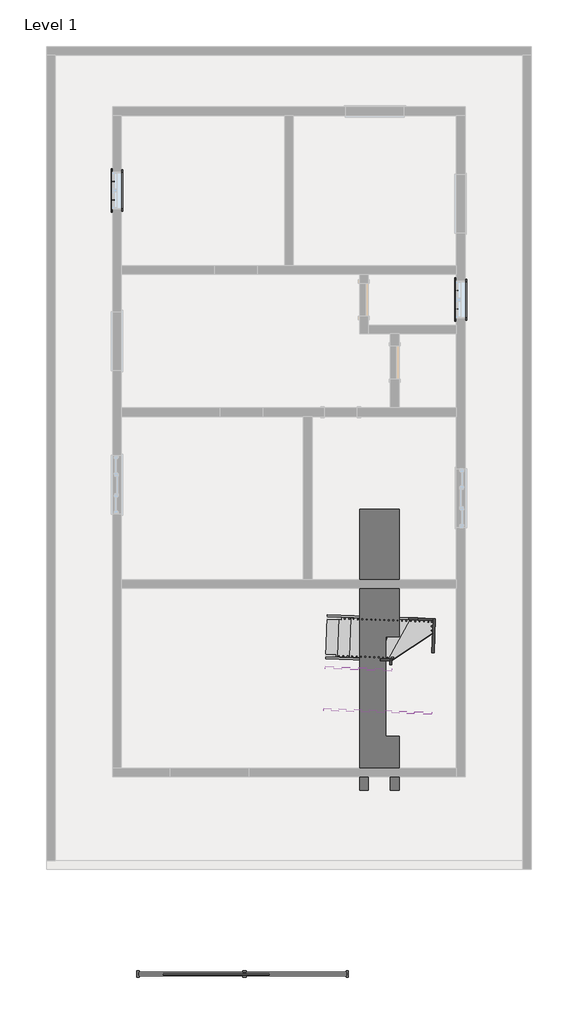
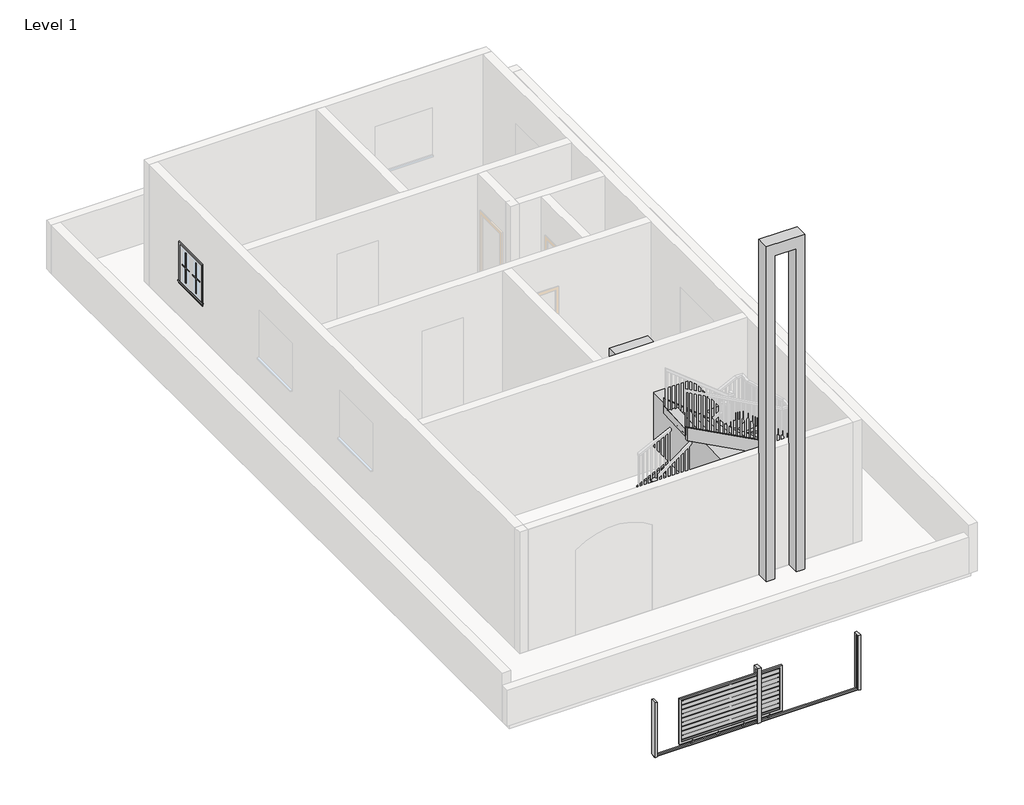
# One storey, part 4 of 4: 18 proxies, 16 members, 2 stair flights, 1 geographic element, 1 railing.
"""IFC4 building model written with IfcOpenShell, lengths in millimetres."""

from ifc_helpers import new_model, si_unit, frame, origin, place, context, project, spatial, polyline, outline, extrude, faceted_brep, transform, mapped, element, save
from components import generic_models_1_generic_models_1_9f30b8ca, generic_models_2_generic_models_2_975c2898, muntin_pattern_2x2_muntin_pattern_2x2_b3fe6957, muntin_pattern_2x2_muntin_pattern_2x2_3e0ecaf2, trim_window_exterior_flat_with_sill_41619996, trim_window_interior_flat_picture_frame_51c85655, sliding_gate_17236_sliding_gate_17236_fdb57db6, stair_flight_9054a24f

model = new_model("IFC4")

# Units and contexts
model_context = context("Model", 3, world=origin())
ifc_project = project(units=[si_unit("LENGTHUNIT", "METRE", prefix="MILLI")], contexts=[model_context])

# Site, building, storey
site = spatial("IfcSite", under=ifc_project)
building = spatial("IfcBuilding", under=site)
storey = spatial("IfcBuildingStorey", under=building, Name="Level 1", Elevation=0.0)

# Proxies
placement = place(None, origin())
generic_models_1_generic_models_1_shape = generic_models_1_generic_models_1_9f30b8ca(model_context)
element("IfcBuildingElementProxy", 1, Name="Generic Models 1 : Generic Models 1", ObjectType="Generic Models 1 : Generic Models 1", at=placement, inside=storey, context=model_context, shape_type="MappedRepresentation", body=[
    mapped(generic_models_1_generic_models_1_shape, transform((0.0, 0.0, 0.0), x_axis=(1.0, 0.0, 0.0), y_axis=(0.0, 1.0, 0.0), z_axis=(0.0, 0.0, 1.0))),
])
generic_models_2_generic_models_2_shape = generic_models_2_generic_models_2_975c2898(model_context)
element("IfcBuildingElementProxy", 2, Name="Generic Models 2 : Generic Models 2", ObjectType="Generic Models 2 : Generic Models 2", at=placement, inside=storey, context=model_context, shape_type="MappedRepresentation", body=[
    mapped(generic_models_2_generic_models_2_shape, transform((0.0, 0.0, 0.0), x_axis=(1.0, 0.0, 0.0), y_axis=(0.0, 1.0, 0.0), z_axis=(0.0, 0.0, 1.0))),
])
muntin_pattern_2x2_muntin_pattern_2x2_shape = muntin_pattern_2x2_muntin_pattern_2x2_b3fe6957(model_context)
element("IfcBuildingElementProxy", 3, Name="Muntin Pattern_2x2 : Muntin Pattern_2x2", ObjectType="Muntin Pattern_2x2 : Muntin Pattern_2x2", at=placement, inside=storey, context=model_context, shape_type="MappedRepresentation", body=[
    mapped(muntin_pattern_2x2_muntin_pattern_2x2_shape, transform((-14939.9876504, 9248.016357, 984.25), x_axis=(0.0, 1.0, 0.0), y_axis=(-1.0, 0.0, 0.0), z_axis=(0.0, 0.0, 1.0))),
])
element("IfcBuildingElementProxy", 4, Name="Muntin Pattern_2x2 : Muntin Pattern_2x2", ObjectType="Muntin Pattern_2x2 : Muntin Pattern_2x2", at=placement, inside=storey, context=model_context, shape_type="MappedRepresentation", body=[
    mapped(muntin_pattern_2x2_muntin_pattern_2x2_shape, transform((-7015.1876504, 6733.416357, 984.25), x_axis=(0.0, 1.0, 0.0), y_axis=(-1.0, 0.0, 0.0), z_axis=(0.0, 0.0, 1.0))),
])
element("IfcBuildingElementProxy", 5, Name="Muntin Pattern_2x2 : Muntin Pattern_2x2", ObjectType="Muntin Pattern_2x2 : Muntin Pattern_2x2", at=placement, inside=storey, context=model_context, shape_type="MappedRepresentation", body=[
    mapped(muntin_pattern_2x2_muntin_pattern_2x2_shape, transform((-14939.9876504, 9248.016357, 984.25), x_axis=(0.0, 1.0, 0.0), y_axis=(-1.0, 0.0, 0.0), z_axis=(0.0, 0.0, 1.0))),
])
element("IfcBuildingElementProxy", 6, Name="Muntin Pattern_2x2 : Muntin Pattern_2x2", ObjectType="Muntin Pattern_2x2 : Muntin Pattern_2x2", at=placement, inside=storey, context=model_context, shape_type="MappedRepresentation", body=[
    mapped(muntin_pattern_2x2_muntin_pattern_2x2_shape, transform((-7015.1876504, 6733.416357, 984.25), x_axis=(0.0, 1.0, 0.0), y_axis=(-1.0, 0.0, 0.0), z_axis=(0.0, 0.0, 1.0))),
])
muntin_pattern_2x2_muntin_pattern_2x2_2_shape = muntin_pattern_2x2_muntin_pattern_2x2_3e0ecaf2(model_context)
element("IfcBuildingElementProxy", 7, Name="Muntin Pattern_2x2 : Muntin Pattern_2x2", ObjectType="Muntin Pattern_2x2 : Muntin Pattern_2x2", at=placement, inside=storey, context=model_context, shape_type="MappedRepresentation", body=[
    mapped(muntin_pattern_2x2_muntin_pattern_2x2_2_shape, transform((-14939.9876504, 9676.641357, 984.25), x_axis=(0.0, -1.0, 0.0), y_axis=(1.0, 0.0, 0.0), z_axis=(0.0, 0.0, 1.0))),
])
element("IfcBuildingElementProxy", 8, Name="Muntin Pattern_2x2 : Muntin Pattern_2x2", ObjectType="Muntin Pattern_2x2 : Muntin Pattern_2x2", at=placement, inside=storey, context=model_context, shape_type="MappedRepresentation", body=[
    mapped(muntin_pattern_2x2_muntin_pattern_2x2_2_shape, transform((-7015.1876504, 7162.041357, 984.25), x_axis=(0.0, -1.0, 0.0), y_axis=(1.0, 0.0, 0.0), z_axis=(0.0, 0.0, 1.0))),
])
element("IfcBuildingElementProxy", 9, Name="Muntin Pattern_2x2 : Muntin Pattern_2x2", ObjectType="Muntin Pattern_2x2 : Muntin Pattern_2x2", at=placement, inside=storey, context=model_context, shape_type="MappedRepresentation", body=[
    mapped(muntin_pattern_2x2_muntin_pattern_2x2_2_shape, transform((-14939.9876504, 9676.641357, 984.25), x_axis=(0.0, -1.0, 0.0), y_axis=(1.0, 0.0, 0.0), z_axis=(0.0, 0.0, 1.0))),
])
element("IfcBuildingElementProxy", 10, Name="Muntin Pattern_2x2 : Muntin Pattern_2x2", ObjectType="Muntin Pattern_2x2 : Muntin Pattern_2x2", at=placement, inside=storey, context=model_context, shape_type="MappedRepresentation", body=[
    mapped(muntin_pattern_2x2_muntin_pattern_2x2_2_shape, transform((-7015.1876504, 7162.041357, 984.25), x_axis=(0.0, -1.0, 0.0), y_axis=(1.0, 0.0, 0.0), z_axis=(0.0, 0.0, 1.0))),
])
trim_window_exterior_flat_with_sill_shape = trim_window_exterior_flat_with_sill_41619996(model_context)
element("IfcBuildingElementProxy", 11, Name="Trim-Window-Exterior-Flat : with Sill", ObjectType="Trim-Window-Exterior-Flat : with Sill", at=placement, inside=storey, context=model_context, shape_type="MappedRepresentation", body=[
    mapped(trim_window_exterior_flat_with_sill_shape, transform((-14949.5126504, 9462.328857, 1828.8), x_axis=(0.0, -1.0, 0.0), y_axis=(0.0, 0.0, 1.0), z_axis=(-1.0, 0.0, 0.0))),
])
element("IfcBuildingElementProxy", 12, Name="Trim-Window-Exterior-Flat : with Sill", ObjectType="Trim-Window-Exterior-Flat : with Sill", at=placement, inside=storey, context=model_context, shape_type="MappedRepresentation", body=[
    mapped(trim_window_exterior_flat_with_sill_shape, transform((-7024.7126504, 6947.728857, 1828.8), x_axis=(0.0, -1.0, 0.0), y_axis=(0.0, 0.0, 1.0), z_axis=(-1.0, 0.0, 0.0))),
])
element("IfcBuildingElementProxy", 13, Name="Trim-Window-Exterior-Flat : with Sill", ObjectType="Trim-Window-Exterior-Flat : with Sill", at=placement, inside=storey, context=model_context, shape_type="MappedRepresentation", body=[
    mapped(trim_window_exterior_flat_with_sill_shape, transform((-14949.5126504, 9462.328857, 1828.8), x_axis=(0.0, -1.0, 0.0), y_axis=(0.0, 0.0, 1.0), z_axis=(-1.0, 0.0, 0.0))),
])
element("IfcBuildingElementProxy", 14, Name="Trim-Window-Exterior-Flat : with Sill", ObjectType="Trim-Window-Exterior-Flat : with Sill", at=placement, inside=storey, context=model_context, shape_type="MappedRepresentation", body=[
    mapped(trim_window_exterior_flat_with_sill_shape, transform((-7024.7126504, 6947.728857, 1828.8), x_axis=(0.0, -1.0, 0.0), y_axis=(0.0, 0.0, 1.0), z_axis=(-1.0, 0.0, 0.0))),
])
trim_window_interior_flat_picture_frame_shape = trim_window_interior_flat_picture_frame_51c85655(model_context)
element("IfcBuildingElementProxy", 15, Name="Trim-Window-Interior-Flat : Picture Frame", ObjectType="Trim-Window-Interior-Flat : Picture Frame", at=placement, inside=storey, context=model_context, shape_type="MappedRepresentation", body=[
    mapped(trim_window_interior_flat_picture_frame_shape, transform((-14746.3126504, 9462.328857, 1828.8), x_axis=(0.0, 1.0, 0.0), y_axis=(0.0, 0.0, 1.0), z_axis=(1.0, 0.0, 0.0))),
])
element("IfcBuildingElementProxy", 16, Name="Trim-Window-Interior-Flat : Picture Frame", ObjectType="Trim-Window-Interior-Flat : Picture Frame", at=placement, inside=storey, context=model_context, shape_type="MappedRepresentation", body=[
    mapped(trim_window_interior_flat_picture_frame_shape, transform((-6821.5126504, 6947.728857, 1828.8), x_axis=(0.0, 1.0, 0.0), y_axis=(0.0, 0.0, 1.0), z_axis=(1.0, 0.0, 0.0))),
])
element("IfcBuildingElementProxy", 17, Name="Trim-Window-Interior-Flat : Picture Frame", ObjectType="Trim-Window-Interior-Flat : Picture Frame", at=placement, inside=storey, context=model_context, shape_type="MappedRepresentation", body=[
    mapped(trim_window_interior_flat_picture_frame_shape, transform((-14746.3126504, 9462.328857, 1828.8), x_axis=(0.0, 1.0, 0.0), y_axis=(0.0, 0.0, 1.0), z_axis=(1.0, 0.0, 0.0))),
])
element("IfcBuildingElementProxy", 18, Name="Trim-Window-Interior-Flat : Picture Frame", ObjectType="Trim-Window-Interior-Flat : Picture Frame", at=placement, inside=storey, context=model_context, shape_type="MappedRepresentation", body=[
    mapped(trim_window_interior_flat_picture_frame_shape, transform((-6821.5126504, 6947.728857, 1828.8), x_axis=(0.0, 1.0, 0.0), y_axis=(0.0, 0.0, 1.0), z_axis=(1.0, 0.0, 0.0))),
])

# Geographic element
sliding_gate_17236_sliding_gate_17236_shape = sliding_gate_17236_sliding_gate_17236_fdb57db6(model_context)
element("IfcGeographicElement", 19, ObjectType="Sliding_Gate_17236 : Sliding_Gate_17236", at=placement, inside=storey, context=model_context, shape_type="MappedRepresentation", body=[
    mapped(sliding_gate_17236_sliding_gate_17236_shape, transform((-14390.7126504, -8673.271143, 0.0), x_axis=(1.0, 0.0, 0.0), y_axis=(0.0, 1.0, 0.0), z_axis=(0.0, 0.0, 1.0))),
])

# Members
element("IfcMember", 20, ObjectType="Stringer - 2\" Width", at=placement, inside=storey, context=model_context, shape_type="SweptSolid", body=[
    extrude(outline(polyline([(157.0794453, -304.8), (51.8818925, -100.6726296), (247.2290139, 0.0), (2348.3102094, 0.0), (2505.3896547, -304.8), (157.0794453, -304.8)])), frame((-10006.394185, -363.3128759, -113.2550622), z_axis=(0.03595828761805287, 0.9993532916599501, 0.0), x_axis=(0.8883269481492083, -0.03196338688929392, 0.45809777896261317)), (0.0, 0.0, 1.0), 50.8),
])
element("IfcMember", 21, ObjectType="Stringer - 2\" Width", at=placement, inside=storey, context=model_context, shape_type="SweptSolid", body=[
    extrude(outline(polyline([(-7920.3269434, -438.3728236), (-7918.5002624, -387.6056764), (-7564.0151591, -400.3606025), (-7565.8418401, -451.1277497), (-7920.3269434, -438.3728236)])), frame((0.0, 0.0, 962.500629), z_axis=(0.0, 0.0, 1.0), x_axis=(1.0, 0.0, 0.0)), (0.0, 0.0, 1.0), 342.8950162),
])
element("IfcMember", 22, ObjectType="Stringer - 2\" Width", at=placement, inside=storey, context=model_context, shape_type="SweptSolid", body=[
    extrude(outline(polyline([(-141.4966894, -274.7041443), (-53.351137, 0.0), (2175.2349578, 0.0), (2210.4467651, -11.2985708), (2109.3071449, -326.4985112), (19.9195916, -326.4985112), (-141.4966894, -274.7041443)])), frame((-7515.0746928, -452.9544307, 1305.3956453), z_axis=(-0.9993532916599502, 0.035958287618053086, 0.0), x_axis=(-0.034238839346999, -0.9515663584286188, 0.30553095978487654)), (0.0, 0.0, 1.0), 50.8),
])
element("IfcMember", 23, ObjectType="Stringer - 2\" Width", at=placement, inside=storey, context=model_context, shape_type="SweptSolid", body=[
    extrude(outline(polyline([(-7590.8819548, -2559.7910402), (-7592.7086358, -2610.5581874), (-7997.9608864, -2595.9765803), (-7996.1342054, -2545.2094331), (-7590.8819548, -2559.7910402)])), frame((0.0, 0.0, 1649.8904473), z_axis=(0.0, 0.0, 1.0), x_axis=(1.0, 0.0, 0.0)), (0.0, 0.0, 1.0), 320.1068224),
])
element("IfcMember", 24, ObjectType="Stringer - 2\" Width", at=placement, inside=storey, context=model_context, shape_type="SweptSolid", body=[
    extrude(outline(polyline([(-146.6402244, -284.5435333), (0.0, 0.0), (2348.3102094, 0.0), (2201.669985, -284.5435333), (-146.6402244, -284.5435333)])), frame((-7997.9608864, -2595.9765803, 1969.9972697), z_axis=(0.03595828761805282, 0.9993532916599503, 0.0), x_axis=(-0.8883269481492089, 0.031963386889293885, 0.45809777896261206)), (0.0, 0.0, 1.0), 50.8),
])
element("IfcMember", 25, ObjectType="Stringer - 2\" Width", at=placement, inside=storey, context=model_context, shape_type="SweptSolid", body=[
    extrude(outline(polyline([(248.5240347, -304.8), (137.1927864, -168.2588219), (343.5522597, 0.0), (1905.6564494, 0.0), (2154.1804842, -304.8), (248.5240347, -304.8)])), frame((-10041.1011242, -1327.888673, -217.1011096), z_axis=(0.03595828761805293, 0.9993532916599501, 0.0), x_axis=(0.7745239433168307, -0.02786857756239004, 0.6319303787709498)), (0.0, 0.0, 1.0), 50.8),
])
element("IfcMember", 26, ObjectType="Stringer - 2\" Width", at=placement, inside=storey, context=model_context, shape_type="SweptSolid", body=[
    extrude(outline(polyline([(-470.0446027, -275.2513009), (0.0, 0.0), (408.9230004, 1e-07), (420.0212921, -18.9524702), (-68.1184117, -304.7999999), (-452.7413132, -304.8), (-470.0446027, -275.2513009)])), frame((-8512.5307482, -1332.0561414, 1573.2682978), z_axis=(-0.9993532916599503, 0.03595828761805069, 0.0), x_axis=(-0.01817045481332337, -0.5049935642524205, 0.8629318250218342)), (0.0, 0.0, 1.0), 50.8),
])
element("IfcMember", 27, ObjectType="Stringer - 2\" Width", at=placement, inside=storey, context=model_context, shape_type="SweptSolid", body=[
    extrude(outline(polyline([(-248.5240348, -304.8), (0.0, 0.0), (1971.2027087, 0.0), (1722.6786739, -304.8), (-248.5240348, -304.8)])), frame((-8522.5774937, -1611.2754511, 1926.1409689), z_axis=(0.0359582876180528, 0.9993532916599502, 0.0), x_axis=(-0.7745239433168302, 0.027868577562389925, 0.6319303787709503)), (0.0, 0.0, 1.0), 50.8),
])
element("IfcMember", 28, ObjectType="Stringer - 2\" Width", at=placement, inside=storey, context=model_context, shape_type="SweptSolid", body=[
    extrude(outline(polyline([(157.0794453, -304.8), (51.8818925, -100.6726296), (247.2290139, 0.0), (2348.3102094, 0.0), (2505.3896547, -304.8), (157.0794453, -304.8)])), frame((-10006.394185, -363.3128759, -113.2550622), z_axis=(0.03595828761805287, 0.9993532916599501, 0.0), x_axis=(0.8883269481492083, -0.03196338688929392, 0.45809777896261317)), (0.0, 0.0, 1.0), 50.8),
])
element("IfcMember", 29, ObjectType="Stringer - 2\" Width", at=placement, inside=storey, context=model_context, shape_type="SweptSolid", body=[
    extrude(outline(polyline([(-7920.3269434, -438.3728236), (-7918.5002624, -387.6056764), (-7564.0151591, -400.3606025), (-7565.8418401, -451.1277497), (-7920.3269434, -438.3728236)])), frame((0.0, 0.0, 962.500629), z_axis=(0.0, 0.0, 1.0), x_axis=(1.0, 0.0, 0.0)), (0.0, 0.0, 1.0), 342.8950162),
])
element("IfcMember", 30, ObjectType="Stringer - 2\" Width", at=placement, inside=storey, context=model_context, shape_type="SweptSolid", body=[
    extrude(outline(polyline([(-141.4966894, -274.7041443), (-53.351137, 0.0), (2175.2349578, 0.0), (2210.4467651, -11.2985708), (2109.3071449, -326.4985112), (19.9195916, -326.4985112), (-141.4966894, -274.7041443)])), frame((-7515.0746928, -452.9544307, 1305.3956453), z_axis=(-0.9993532916599502, 0.035958287618053086, 0.0), x_axis=(-0.034238839346999, -0.9515663584286188, 0.30553095978487654)), (0.0, 0.0, 1.0), 50.8),
])
element("IfcMember", 31, ObjectType="Stringer - 2\" Width", at=placement, inside=storey, context=model_context, shape_type="SweptSolid", body=[
    extrude(outline(polyline([(-7590.8819548, -2559.7910402), (-7592.7086358, -2610.5581874), (-7997.9608864, -2595.9765803), (-7996.1342054, -2545.2094331), (-7590.8819548, -2559.7910402)])), frame((0.0, 0.0, 1649.8904473), z_axis=(0.0, 0.0, 1.0), x_axis=(1.0, 0.0, 0.0)), (0.0, 0.0, 1.0), 320.1068224),
])
element("IfcMember", 32, ObjectType="Stringer - 2\" Width", at=placement, inside=storey, context=model_context, shape_type="SweptSolid", body=[
    extrude(outline(polyline([(-146.6402244, -284.5435333), (0.0, 0.0), (2348.3102094, 0.0), (2201.669985, -284.5435333), (-146.6402244, -284.5435333)])), frame((-7997.9608864, -2595.9765803, 1969.9972697), z_axis=(0.03595828761805282, 0.9993532916599503, 0.0), x_axis=(-0.8883269481492089, 0.031963386889293885, 0.45809777896261206)), (0.0, 0.0, 1.0), 50.8),
])
element("IfcMember", 33, ObjectType="Stringer - 2\" Width", at=placement, inside=storey, context=model_context, shape_type="SweptSolid", body=[
    extrude(outline(polyline([(248.5240347, -304.8), (137.1927864, -168.2588219), (343.5522597, 0.0), (1905.6564494, 0.0), (2154.1804842, -304.8), (248.5240347, -304.8)])), frame((-10041.1011242, -1327.888673, -217.1011096), z_axis=(0.03595828761805293, 0.9993532916599501, 0.0), x_axis=(0.7745239433168307, -0.02786857756239004, 0.6319303787709498)), (0.0, 0.0, 1.0), 50.8),
])
element("IfcMember", 34, ObjectType="Stringer - 2\" Width", at=placement, inside=storey, context=model_context, shape_type="SweptSolid", body=[
    extrude(outline(polyline([(-470.0446027, -275.2513009), (0.0, 0.0), (408.9230004, 1e-07), (420.0212921, -18.9524702), (-68.1184117, -304.7999999), (-452.7413132, -304.8), (-470.0446027, -275.2513009)])), frame((-8512.5307482, -1332.0561414, 1573.2682978), z_axis=(-0.9993532916599503, 0.03595828761805069, 0.0), x_axis=(-0.01817045481332337, -0.5049935642524205, 0.8629318250218342)), (0.0, 0.0, 1.0), 50.8),
])
element("IfcMember", 35, ObjectType="Stringer - 2\" Width", at=placement, inside=storey, context=model_context, shape_type="SweptSolid", body=[
    extrude(outline(polyline([(-248.5240348, -304.8), (0.0, 0.0), (1971.2027087, 0.0), (1722.6786739, -304.8), (-248.5240348, -304.8)])), frame((-8522.5774937, -1611.2754511, 1926.1409689), z_axis=(0.0359582876180528, 0.9993532916599502, 0.0), x_axis=(-0.7745239433168302, 0.027868577562389925, 0.6319303787709503)), (0.0, 0.0, 1.0), 50.8),
])

# Railing
element("IfcRailing", 36, ObjectType="Handrail - Rectangular", at=placement, inside=storey, context=model_context, shape_type="SolidModel", body=[
    faceted_brep([(-10006.394185, -363.3128759, 1083.7333333), (-10006.394185, -363.3128759, 1026.2742652), (-10008.220866, -414.0800231, 1026.2742652), (-10008.220866, -414.0800231, 1083.7333333), (-7750.1292126, -444.496803, 2277.0239201), (-7737.5382959, -444.9498438, 2226.2239201), (-7739.364977, -495.716991, 2226.2239201), (-7751.9558936, -495.2639503, 2277.0239201), (-7565.8418401, -451.1277497, 2277.0239201), (-7565.8418401, -451.1277497, 2226.2239201), (-7618.4356683, -500.0682159, 2226.2239201), (-7618.4356683, -500.0682159, 2277.0239201), (-7576.1730834, -738.2538248, 2277.0239201), (-7576.4589725, -746.1992592, 2226.2239201), (-7627.2261197, -744.3725782, 2226.2239201), (-7626.9402306, -736.4271438, 2277.0239201), (-7631.3178587, -2270.838284, 2769.1094132), (-7631.6037478, -2278.7837184, 2718.3094132), (-7682.370895, -2276.9570374, 2718.3094132), (-7682.0850059, -2269.011603, 2769.1094132), (-7641.649102, -2557.9643591, 2769.1094132), (-7641.649102, -2557.9643591, 2718.3094132), (-7690.5895682, -2505.3705309, 2718.3094132), (-7690.5895682, -2505.3705309, 2769.1094132), (-7825.9364745, -2551.3334125, 2769.1094132), (-7838.5273911, -2550.8803717, 2718.3094132), (-7836.7007101, -2500.1132245, 2718.3094132), (-7824.1097935, -2500.5662653, 2769.1094132), (-10082.2014469, -2470.1494854, 3962.4), (-10080.3747659, -2419.3823382, 3962.4), (-10080.3747659, -2419.3823382, 3904.9409318), (-10082.2014469, -2470.1494854, 3904.9409318)], [[[0, 1, 2, 3]], [[1, 0, 4, 5]], [[2, 1, 5, 6]], [[3, 2, 6, 7]], [[0, 3, 7, 4]], [[5, 4, 8, 9]], [[6, 5, 9, 10]], [[7, 6, 10, 11]], [[4, 7, 11, 8]], [[9, 8, 12, 13]], [[10, 9, 13, 14]], [[11, 10, 14, 15]], [[8, 11, 15, 12]], [[13, 12, 16, 17]], [[14, 13, 17, 18]], [[15, 14, 18, 19]], [[12, 15, 19, 16]], [[17, 16, 20, 21]], [[18, 17, 21, 22]], [[19, 18, 22, 23]], [[16, 19, 23, 20]], [[21, 20, 24, 25]], [[22, 21, 25, 26]], [[23, 22, 26, 27]], [[20, 23, 27, 24]], [[28, 29, 30, 31]], [[25, 24, 28, 31]], [[26, 25, 31, 30]], [[27, 26, 30, 29]], [[24, 27, 29, 28]]]),
    extrude(outline(polyline([(223.5656878, 19.05), (1212.6274313, 19.05), (1212.6274313, 0.0), (233.6343122, 0.0), (223.5656878, 19.05)])), frame((-9992.2317697, -2457.5014613, 4091.294098), z_axis=(0.035958287618052934, 0.9993532916599503, 0.0), x_axis=(0.0, 0.0, -1.0)), (0.0, 0.0, 1.0), 19.05),
    extrude(outline(polyline([(223.5656878, 19.05), (1158.9281011, 19.05), (1158.9281011, 0.0), (233.6343122, 0.0), (223.5656878, 19.05)])), frame((-9890.6974752, -2461.1548233, 4037.5947678), z_axis=(0.035958287618052934, 0.9993532916599503, 0.0), x_axis=(0.0, 0.0, -1.0)), (0.0, 0.0, 1.0), 19.05),
    extrude(outline(polyline([(223.5656878, 19.05), (1274.5621043, 19.05), (1274.5621043, 0.0), (233.6343122, 0.0), (223.5656878, 19.05)])), frame((-9789.1631808, -2464.8081854, 3983.8954376), z_axis=(0.035958287618052934, 0.9993532916599503, 0.0), x_axis=(0.0, 0.0, -1.0)), (0.0, 0.0, 1.0), 19.05),
    extrude(outline(polyline([(223.5656878, 19.05), (1220.8627741, 19.05), (1220.8627741, 0.0), (233.6343122, 0.0), (223.5656878, 19.05)])), frame((-9687.6288864, -2468.4615474, 3930.1961074), z_axis=(0.035958287618052934, 0.9993532916599503, 0.0), x_axis=(0.0, 0.0, -1.0)), (0.0, 0.0, 1.0), 19.05),
    extrude(outline(polyline([(223.5656878, 19.05), (1167.1634439, 19.05), (1167.1634439, 0.0), (233.6343122, 0.0), (223.5656878, 19.05)])), frame((-9586.0945919, -2472.1149094, 3876.4967772), z_axis=(0.035958287618052934, 0.9993532916599503, 0.0), x_axis=(0.0, 0.0, -1.0)), (0.0, 0.0, 1.0), 19.05),
    extrude(outline(polyline([(223.5656878, 19.05), (1282.797447, 19.05), (1282.797447, 0.0), (233.6343122, 0.0), (223.5656878, 19.05)])), frame((-9484.5602975, -2475.7682714, 3822.797447), z_axis=(0.035958287618052934, 0.9993532916599503, 0.0), x_axis=(0.0, 0.0, -1.0)), (0.0, 0.0, 1.0), 19.05),
    extrude(outline(polyline([(223.5656878, 19.05), (1229.0981168, 19.05), (1229.0981168, 0.0), (233.6343122, 0.0), (223.5656878, 19.05)])), frame((-9383.0260031, -2479.4216334, 3769.0981168), z_axis=(0.035958287618052934, 0.9993532916599503, 0.0), x_axis=(0.0, 0.0, -1.0)), (0.0, 0.0, 1.0), 19.05),
    extrude(outline(polyline([(223.5656878, 19.05), (1175.3987866, 19.05), (1175.3987866, 0.0), (233.6343122, 0.0), (223.5656878, 19.05)])), frame((-9281.4917086, -2483.0749955, 3715.3987866), z_axis=(0.035958287618052934, 0.9993532916599503, 0.0), x_axis=(0.0, 0.0, -1.0)), (0.0, 0.0, 1.0), 19.05),
    extrude(outline(polyline([(223.5656878, 19.05), (1291.0327897, 19.05), (1291.0327897, 0.0), (233.6343122, 0.0), (223.5656878, 19.05)])), frame((-9179.9574142, -2486.7283575, 3661.6994564), z_axis=(0.035958287618052934, 0.9993532916599503, 0.0), x_axis=(0.0, 0.0, -1.0)), (0.0, 0.0, 1.0), 19.05),
    extrude(outline(polyline([(223.5656878, 19.05), (1237.3334595, 19.05), (1237.3334595, 0.0), (233.6343122, 0.0), (223.5656878, 19.05)])), frame((-9078.4231198, -2490.3817195, 3608.0001262), z_axis=(0.035958287618052934, 0.9993532916599503, 0.0), x_axis=(0.0, 0.0, -1.0)), (0.0, 0.0, 1.0), 19.05),
    extrude(outline(polyline([(223.5656878, 19.05), (1183.6341293, 19.05), (1183.6341293, 0.0), (233.6343122, 0.0), (223.5656878, 19.05)])), frame((-8976.8888253, -2494.0350815, 3554.300796), z_axis=(0.035958287618052934, 0.9993532916599503, 0.0), x_axis=(0.0, 0.0, -1.0)), (0.0, 0.0, 1.0), 19.05),
    extrude(outline(polyline([(223.5656878, 19.05), (1299.2681325, 19.05), (1299.2681325, 0.0), (233.6343122, 0.0), (223.5656878, 19.05)])), frame((-8875.3545309, -2497.6884436, 3500.6014658), z_axis=(0.035958287618052934, 0.9993532916599503, 0.0), x_axis=(0.0, 0.0, -1.0)), (0.0, 0.0, 1.0), 19.05),
    extrude(outline(polyline([(223.5656878, 19.05), (1245.5688023, 19.05), (1245.5688023, 0.0), (233.6343122, 0.0), (223.5656878, 19.05)])), frame((-8773.8202365, -2501.3418056, 3446.9021356), z_axis=(0.035958287618052934, 0.9993532916599503, 0.0), x_axis=(0.0, 0.0, -1.0)), (0.0, 0.0, 1.0), 19.05),
    extrude(outline(polyline([(223.5656878, 19.05), (1191.8694721, 19.05), (1191.8694721, 0.0), (233.6343122, 0.0), (223.5656878, 19.05)])), frame((-8672.285942, -2504.9951676, 3393.2028054), z_axis=(0.035958287618052934, 0.9993532916599503, 0.0), x_axis=(0.0, 0.0, -1.0)), (0.0, 0.0, 1.0), 19.05),
    extrude(outline(polyline([(223.5656878, 19.05), (1138.1701419, 19.05), (1138.1701419, 0.0), (233.6343122, 0.0), (223.5656878, 19.05)])), frame((-8570.7516476, -2508.6485296, 3339.5034752), z_axis=(0.035958287618052934, 0.9993532916599503, 0.0), x_axis=(0.0, 0.0, -1.0)), (0.0, 0.0, 1.0), 19.05),
    extrude(outline(polyline([(223.5656878, 19.05), (1253.804145, 19.05), (1253.804145, 0.0), (233.6343122, 0.0), (223.5656878, 19.05)])), frame((-8469.2173532, -2512.3018916, 3285.804145), z_axis=(0.035958287618052934, 0.9993532916599503, 0.0), x_axis=(0.0, 0.0, -1.0)), (0.0, 0.0, 1.0), 19.05),
    extrude(outline(polyline([(223.5656878, 19.05), (1200.1048148, 19.05), (1200.1048148, 0.0), (233.6343122, 0.0), (223.5656878, 19.05)])), frame((-8367.6830587, -2515.9552537, 3232.1048148), z_axis=(0.035958287618052934, 0.9993532916599503, 0.0), x_axis=(0.0, 0.0, -1.0)), (0.0, 0.0, 1.0), 19.05),
    extrude(outline(polyline([(223.5656878, 19.05), (1146.4054846, 19.05), (1146.4054846, 0.0), (233.6343122, 0.0), (223.5656878, 19.05)])), frame((-8266.1487643, -2519.6086157, 3178.4054846), z_axis=(0.035958287618052934, 0.9993532916599503, 0.0), x_axis=(0.0, 0.0, -1.0)), (0.0, 0.0, 1.0), 19.05),
    extrude(outline(polyline([(223.5656878, 19.05), (1092.7061544, 19.05), (1092.7061544, 0.0), (233.6343122, 0.0), (223.5656878, 19.05)])), frame((-8164.6144699, -2523.2619777, 3124.7061544), z_axis=(0.035958287618052934, 0.9993532916599503, 0.0), x_axis=(0.0, 0.0, -1.0)), (0.0, 0.0, 1.0), 19.05),
    extrude(outline(polyline([(223.5656878, 19.05), (1208.3401575, 19.05), (1208.3401575, 0.0), (233.6343122, 0.0), (223.5656878, 19.05)])), frame((-8063.0801754, -2526.9153397, 3071.0068242), z_axis=(0.035958287618052934, 0.9993532916599503, 0.0), x_axis=(0.0, 0.0, -1.0)), (0.0, 0.0, 1.0), 19.05),
    extrude(outline(polyline([(223.5656878, 19.05), (1154.6408273, 19.05), (1154.6408273, 0.0), (233.6343122, 0.0), (223.5656878, 19.05)])), frame((-7961.545881, -2530.5687018, 3017.307494), z_axis=(0.035958287618052934, 0.9993532916599503, 0.0), x_axis=(0.0, 0.0, -1.0)), (0.0, 0.0, 1.0), 19.05),
    extrude(outline(polyline([(223.5656878, 19.05), (1100.9414971, 19.05), (1100.9414971, 0.0), (233.6343122, 0.0), (223.5656878, 19.05)])), frame((-7860.0115866, -2534.2220638, 2963.6081638), z_axis=(0.035958287618052934, 0.9993532916599503, 0.0), x_axis=(0.0, 0.0, -1.0)), (0.0, 0.0, 1.0), 19.05),
    extrude(outline(polyline([(-7758.4772921, -2537.8754258), (-7777.5149723, -2537.1904204), (-7776.829967, -2518.1527402), (-7757.7922868, -2518.8377456), (-7758.4772921, -2537.8754258)])), frame((0.0, 0.0, 1862.6666667), z_axis=(0.0, 0.0, 1.0), x_axis=(1.0, 0.0, 0.0)), (0.0, 0.0, 1.0), 855.6427466),
    extrude(outline(polyline([(-7655.3446518, -2497.107534), (-7656.0296572, -2516.1452142), (-7675.0673374, -2515.4602088), (-7674.382332, -2496.4225286), (-7655.3446518, -2497.107534)])), frame((0.0, 0.0, 1862.6666667), z_axis=(0.0, 0.0, 1.0), x_axis=(1.0, 0.0, 0.0)), (0.0, 0.0, 1.0), 855.6427466),
    extrude(outline(polyline([(-7651.6912898, -2395.5732396), (-7652.3762952, -2414.6109198), (-7671.4139754, -2413.9259144), (-7670.72897, -2394.8882342), (-7651.6912898, -2395.5732396)])), frame((0.0, 0.0, 1862.6666667), z_axis=(0.0, 0.0, 1.0), x_axis=(1.0, 0.0, 0.0)), (0.0, 0.0, 1.0), 855.6427466),
    extrude(outline(polyline([(-7648.0379278, -2294.0389451), (-7648.7229332, -2313.0766254), (-7667.7606134, -2312.39162), (-7667.075608, -2293.3539398), (-7648.0379278, -2294.0389451)])), frame((0.0, 0.0, 1862.6666667), z_axis=(0.0, 0.0, 1.0), x_axis=(1.0, 0.0, 0.0)), (0.0, 0.0, 1.0), 855.6427466),
    extrude(outline(polyline([(225.5436705, 19.05), (1229.1130279, 19.05), (1229.1130279, 0.0), (231.6563296, 0.0), (225.5436705, 19.05)])), frame((-7644.3845658, -2192.5046507, 2922.4463612), z_axis=(-0.9993532916599501, 0.03595828761805307, 0.0), x_axis=(0.0, 0.0, -1.0)), (0.0, 0.0, 1.0), 19.05),
    extrude(outline(polyline([(225.5436704, 19.05), (1196.5121796, 19.05), (1196.5121796, 0.0), (231.6563295, 0.0), (225.5436704, 19.05)])), frame((-7640.7312037, -2090.9703563, 2889.8455129), z_axis=(-0.9993532916599501, 0.03595828761805307, 0.0), x_axis=(0.0, 0.0, -1.0)), (0.0, 0.0, 1.0), 19.05),
    extrude(outline(polyline([(225.5436705, 19.0500001), (1163.9113314, 19.0500001), (1163.9113314, 0.0), (231.6563295, 0.0), (225.5436705, 19.0500001)])), frame((-7637.0778417, -1989.4360618, 2857.2446647), z_axis=(-0.9993532916599501, 0.03595828761805307, 0.0), x_axis=(0.0, 0.0, -1.0)), (0.0, 0.0, 1.0), 19.05),
    extrude(outline(polyline([(225.5436705, 19.05), (1131.3104832, 19.05), (1131.3104832, 0.0), (231.6563295, 0.0), (225.5436705, 19.05)])), frame((-7633.4244797, -1887.9017674, 2824.6438165), z_axis=(-0.9993532916599501, 0.03595828761805307, 0.0), x_axis=(0.0, 0.0, -1.0)), (0.0, 0.0, 1.0), 19.05),
    extrude(outline(polyline([(225.5436705, 19.05), (1098.709635, 19.05), (1098.709635, 0.0), (231.6563296, 0.0), (225.5436705, 19.05)])), frame((-7629.7711177, -1786.367473, 2792.0429683), z_axis=(-0.9993532916599501, 0.03595828761805307, 0.0), x_axis=(0.0, 0.0, -1.0)), (0.0, 0.0, 1.0), 19.05),
    extrude(outline(polyline([(225.5436705, 19.0500001), (1235.44212, 19.0500001), (1235.44212, 0.0), (231.6563295, 0.0), (225.5436705, 19.0500001)])), frame((-7626.1177556, -1684.8331785, 2759.44212), z_axis=(-0.9993532916599501, 0.03595828761805307, 0.0), x_axis=(0.0, 0.0, -1.0)), (0.0, 0.0, 1.0), 19.05),
    extrude(outline(polyline([(225.5436705, 19.05), (1202.8412718, 19.05), (1202.8412718, 0.0), (231.6563295, 0.0), (225.5436705, 19.05)])), frame((-7622.4643936, -1583.2988841, 2726.8412718), z_axis=(-0.9993532916599501, 0.03595828761805307, 0.0), x_axis=(0.0, 0.0, -1.0)), (0.0, 0.0, 1.0), 19.05),
    extrude(outline(polyline([(225.5436705, 19.05), (1170.2404236, 19.05), (1170.2404236, 0.0), (231.6563295, 0.0), (225.5436705, 19.05)])), frame((-7618.8110316, -1481.7645897, 2694.2404236), z_axis=(-0.9993532916599501, 0.03595828761805307, 0.0), x_axis=(0.0, 0.0, -1.0)), (0.0, 0.0, 1.0), 19.05),
    extrude(outline(polyline([(225.5436704, 19.05), (1137.6395753, 19.05), (1137.6395753, 0.0), (231.6563295, 0.0), (225.5436704, 19.05)])), frame((-7615.1576696, -1380.2302953, 2661.6395753), z_axis=(-0.9993532916599501, 0.03595828761805307, 0.0), x_axis=(0.0, 0.0, -1.0)), (0.0, 0.0, 1.0), 19.05),
    extrude(outline(polyline([(225.5436705, 19.05), (1105.0387271, 19.05), (1105.0387271, 0.0), (231.6563295, 0.0), (225.5436705, 19.05)])), frame((-7611.5043076, -1278.6960008, 2629.0387271), z_axis=(-0.9993532916599501, 0.03595828761805307, 0.0), x_axis=(0.0, 0.0, -1.0)), (0.0, 0.0, 1.0), 19.05),
    extrude(outline(polyline([(225.5436705, 19.05), (1241.7712122, 19.05), (1241.7712122, 0.0), (231.6563295, 0.0), (225.5436705, 19.05)])), frame((-7607.8509455, -1177.1617064, 2596.4378789), z_axis=(-0.9993532916599501, 0.03595828761805307, 0.0), x_axis=(0.0, 0.0, -1.0)), (0.0, 0.0, 1.0), 19.05),
    extrude(outline(polyline([(225.5436705, 19.05), (1209.170364, 19.05), (1209.170364, 0.0), (231.6563296, 0.0), (225.5436705, 19.05)])), frame((-7604.1975835, -1075.627412, 2563.8370307), z_axis=(-0.9993532916599501, 0.03595828761805307, 0.0), x_axis=(0.0, 0.0, -1.0)), (0.0, 0.0, 1.0), 19.05),
    extrude(outline(polyline([(225.5436704, 19.05), (1176.5695157, 19.05), (1176.5695157, 0.0), (231.6563295, 0.0), (225.5436704, 19.05)])), frame((-7600.5442215, -974.0931175, 2531.2361824), z_axis=(-0.9993532916599501, 0.03595828761805307, 0.0), x_axis=(0.0, 0.0, -1.0)), (0.0, 0.0, 1.0), 19.05),
    extrude(outline(polyline([(225.5436705, 19.05), (1143.9686675, 19.05), (1143.9686675, 0.0), (231.6563295, 0.0), (225.5436705, 19.05)])), frame((-7596.8908595, -872.5588231, 2498.6353342), z_axis=(-0.9993532916599501, 0.03595828761805307, 0.0), x_axis=(0.0, 0.0, -1.0)), (0.0, 0.0, 1.0), 19.05),
    extrude(outline(polyline([(225.5436705, 19.05), (1111.3678193, 19.05), (1111.3678193, 0.0), (231.6563295, 0.0), (225.5436705, 19.05)])), frame((-7593.2374974, -771.0245287, 2466.034486), z_axis=(-0.9993532916599501, 0.03595828761805307, 0.0), x_axis=(0.0, 0.0, -1.0)), (0.0, 0.0, 1.0), 19.05),
    extrude(outline(polyline([(-7589.5841354, -669.4902342), (-7590.2691408, -688.5279144), (-7609.306821, -687.842909), (-7608.6218156, -668.8052288), (-7589.5841354, -669.4902342)])), frame((0.0, 0.0, 1185.3333333), z_axis=(0.0, 0.0, 1.0), x_axis=(1.0, 0.0, 0.0)), (0.0, 0.0, 1.0), 1040.8905868),
    extrude(outline(polyline([(-7585.9307734, -567.9559398), (-7586.6157788, -586.99362), (-7605.653459, -586.3086146), (-7604.9684536, -567.2709344), (-7585.9307734, -567.9559398)])), frame((0.0, 0.0, 1185.3333333), z_axis=(0.0, 0.0, 1.0), x_axis=(1.0, 0.0, 0.0)), (0.0, 0.0, 1.0), 1040.8905868),
    extrude(outline(polyline([(-7681.195091, -462.8624332), (-7662.1574108, -463.5474386), (-7662.8424161, -482.5851188), (-7681.8800963, -481.9001134), (-7681.195091, -462.8624332)])), frame((0.0, 0.0, 1185.3333333), z_axis=(0.0, 0.0, 1.0), x_axis=(1.0, 0.0, 0.0)), (0.0, 0.0, 1.0), 1040.8905868),
    extrude(outline(polyline([(233.6343122, 19.05), (1250.9261963, 19.05), (1250.9261963, 0.0), (223.5656878, 0.0), (233.6343122, 19.05)])), frame((-7764.3767106, -478.9317568, 2436.2595296), z_axis=(0.03595828761805286, 0.9993532916599503, 0.0), x_axis=(0.0, 0.0, -1.0)), (0.0, 0.0, 1.0), 19.05),
    extrude(outline(polyline([(233.6343122, 19.05), (1197.2268661, 19.05), (1197.2268661, 0.0), (223.5656878, 0.0), (233.6343122, 19.05)])), frame((-7865.911005, -475.2783948, 2382.5601994), z_axis=(0.03595828761805286, 0.9993532916599503, 0.0), x_axis=(0.0, 0.0, -1.0)), (0.0, 0.0, 1.0), 19.05),
    extrude(outline(polyline([(233.6343122, 19.05), (1143.5275359, 19.05), (1143.5275359, 0.0), (223.5656878, 0.0), (233.6343122, 19.05)])), frame((-7967.4452994, -471.6250327, 2328.8608692), z_axis=(0.03595828761805286, 0.9993532916599503, 0.0), x_axis=(0.0, 0.0, -1.0)), (0.0, 0.0, 1.0), 19.05),
    extrude(outline(polyline([(233.6343122, 19.05), (1089.8282057, 19.05), (1089.8282057, 0.0), (223.5656878, 0.0), (233.6343122, 19.05)])), frame((-8068.9795939, -467.9716707, 2275.161539), z_axis=(0.03595828761805286, 0.9993532916599503, 0.0), x_axis=(0.0, 0.0, -1.0)), (0.0, 0.0, 1.0), 19.05),
    extrude(outline(polyline([(233.6343122, 19.05), (1205.4622088, 19.05), (1205.4622088, 0.0), (223.5656878, 0.0), (233.6343122, 19.05)])), frame((-8170.5138883, -464.3183087, 2221.4622088), z_axis=(0.03595828761805286, 0.9993532916599503, 0.0), x_axis=(0.0, 0.0, -1.0)), (0.0, 0.0, 1.0), 19.05),
    extrude(outline(polyline([(233.6343122, 19.05), (1151.7628786, 19.05), (1151.7628786, 0.0), (223.5656878, 0.0), (233.6343122, 19.05)])), frame((-8272.0481827, -460.6649467, 2167.7628786), z_axis=(0.03595828761805286, 0.9993532916599503, 0.0), x_axis=(0.0, 0.0, -1.0)), (0.0, 0.0, 1.0), 19.05),
    extrude(outline(polyline([(233.6343122, 19.05), (1098.0635484, 19.05), (1098.0635484, 0.0), (223.5656878, 0.0), (233.6343122, 19.05)])), frame((-8373.5824772, -457.0115846, 2114.0635484), z_axis=(0.03595828761805286, 0.9993532916599503, 0.0), x_axis=(0.0, 0.0, -1.0)), (0.0, 0.0, 1.0), 19.05),
    extrude(outline(polyline([(233.6343122, 19.05), (1044.3642182, 19.05), (1044.3642182, 0.0), (223.5656878, 0.0), (233.6343122, 19.05)])), frame((-8475.1167716, -453.3582226, 2060.3642182), z_axis=(0.03595828761805286, 0.9993532916599503, 0.0), x_axis=(0.0, 0.0, -1.0)), (0.0, 0.0, 1.0), 19.05),
    extrude(outline(polyline([(233.6343122, 19.05), (1159.9982213, 19.05), (1159.9982213, 0.0), (223.5656878, 0.0), (233.6343122, 19.05)])), frame((-8576.651066, -449.7048606, 2006.664888), z_axis=(0.03595828761805286, 0.9993532916599503, 0.0), x_axis=(0.0, 0.0, -1.0)), (0.0, 0.0, 1.0), 19.05),
    extrude(outline(polyline([(233.6343122, 19.05), (1106.2988911, 19.05), (1106.2988911, 0.0), (223.5656878, 0.0), (233.6343122, 19.05)])), frame((-8678.1853605, -446.0514986, 1952.9655578), z_axis=(0.03595828761805286, 0.9993532916599503, 0.0), x_axis=(0.0, 0.0, -1.0)), (0.0, 0.0, 1.0), 19.05),
    extrude(outline(polyline([(233.6343122, 19.05), (1052.5995609, 19.05), (1052.5995609, 0.0), (223.5656878, 0.0), (233.6343122, 19.05)])), frame((-8779.7196549, -442.3981366, 1899.2662276), z_axis=(0.03595828761805286, 0.9993532916599503, 0.0), x_axis=(0.0, 0.0, -1.0)), (0.0, 0.0, 1.0), 19.05),
    extrude(outline(polyline([(233.6343122, 19.05), (1168.2335641, 19.05), (1168.2335641, 0.0), (223.5656878, 0.0), (233.6343122, 19.05)])), frame((-8881.2539493, -438.7447745, 1845.5668974), z_axis=(0.03595828761805286, 0.9993532916599503, 0.0), x_axis=(0.0, 0.0, -1.0)), (0.0, 0.0, 1.0), 19.05),
    extrude(outline(polyline([(233.6343122, 19.05), (1114.5342339, 19.05), (1114.5342339, 0.0), (223.5656878, 0.0), (233.6343122, 19.05)])), frame((-8982.7882438, -435.0914125, 1791.8675672), z_axis=(0.03595828761805286, 0.9993532916599503, 0.0), x_axis=(0.0, 0.0, -1.0)), (0.0, 0.0, 1.0), 19.05),
    extrude(outline(polyline([(233.6343122, 19.05), (1060.8349037, 19.05), (1060.8349037, 0.0), (223.5656878, 0.0), (233.6343122, 19.05)])), frame((-9084.3225382, -431.4380505, 1738.168237), z_axis=(0.03595828761805286, 0.9993532916599503, 0.0), x_axis=(0.0, 0.0, -1.0)), (0.0, 0.0, 1.0), 19.05),
    extrude(outline(polyline([(233.6343122, 19.05), (1176.4689068, 19.05), (1176.4689068, 0.0), (223.5656878, 0.0), (233.6343122, 19.05)])), frame((-9185.8568326, -427.7846885, 1684.4689068), z_axis=(0.03595828761805286, 0.9993532916599503, 0.0), x_axis=(0.0, 0.0, -1.0)), (0.0, 0.0, 1.0), 19.05),
    extrude(outline(polyline([(233.6343122, 19.05), (1122.7695766, 19.05), (1122.7695766, 0.0), (223.5656878, 0.0), (233.6343122, 19.05)])), frame((-9287.3911271, -424.1313264, 1630.7695766), z_axis=(0.03595828761805286, 0.9993532916599503, 0.0), x_axis=(0.0, 0.0, -1.0)), (0.0, 0.0, 1.0), 19.05),
    extrude(outline(polyline([(233.6343122, 19.05), (1069.0702464, 19.05), (1069.0702464, 0.0), (223.5656878, 0.0), (233.6343122, 19.05)])), frame((-9388.9254215, -420.4779644, 1577.0702464), z_axis=(0.03595828761805286, 0.9993532916599503, 0.0), x_axis=(0.0, 0.0, -1.0)), (0.0, 0.0, 1.0), 19.05),
    extrude(outline(polyline([(233.6343122, 19.05), (1184.7042495, 19.05), (1184.7042495, 0.0), (223.5656878, 0.0), (233.6343122, 19.05)])), frame((-9490.4597159, -416.8246024, 1523.3709162), z_axis=(0.03595828761805286, 0.9993532916599503, 0.0), x_axis=(0.0, 0.0, -1.0)), (0.0, 0.0, 1.0), 19.05),
    extrude(outline(polyline([(233.6343122, 19.05), (1131.0049193, 19.05), (1131.0049193, 0.0), (223.5656878, 0.0), (233.6343122, 19.05)])), frame((-9591.9940104, -413.1712404, 1469.671586), z_axis=(0.03595828761805286, 0.9993532916599503, 0.0), x_axis=(0.0, 0.0, -1.0)), (0.0, 0.0, 1.0), 19.05),
    extrude(outline(polyline([(233.6343122, 19.05), (1077.3055891, 19.05), (1077.3055891, 0.0), (223.5656878, 0.0), (233.6343122, 19.05)])), frame((-9693.5283048, -409.5178784, 1415.9722558), z_axis=(0.03595828761805286, 0.9993532916599503, 0.0), x_axis=(0.0, 0.0, -1.0)), (0.0, 0.0, 1.0), 19.05),
    extrude(outline(polyline([(233.6343122, 19.05), (1192.9395923, 19.05), (1192.9395923, 0.0), (223.5656878, 0.0), (233.6343122, 19.05)])), frame((-9795.0625992, -405.8645163, 1362.2729256), z_axis=(0.03595828761805286, 0.9993532916599503, 0.0), x_axis=(0.0, 0.0, -1.0)), (0.0, 0.0, 1.0), 19.05),
    extrude(outline(polyline([(233.6343123, 19.0500001), (1139.2402621, 19.0500001), (1139.2402621, 0.0), (223.5656878, 0.0), (233.6343123, 19.0500001)])), frame((-9896.5968936, -402.2111543, 1308.5735954), z_axis=(0.03595828761805286, 0.9993532916599503, 0.0), x_axis=(0.0, 0.0, -1.0)), (0.0, 0.0, 1.0), 19.05),
    extrude(outline(polyline([(-7656.2579923, -2522.4911076), (-7656.9429977, -2541.5287878), (-7675.9806779, -2540.8437824), (-7675.2956725, -2521.8061022), (-7656.2579923, -2522.4911076)])), frame((0.0, 0.0, 1862.6666667), z_axis=(0.0, 0.0, 1.0), x_axis=(1.0, 0.0, 0.0)), (0.0, 0.0, 1.0), 855.6427466),
    extrude(outline(polyline([(-7601.3150916, -465.73664), (-7582.2774114, -466.4216454), (-7582.9624168, -485.4593256), (-7602.000097, -484.7743202), (-7601.3150916, -465.73664)])), frame((0.0, 0.0, 1185.3333333), z_axis=(0.0, 0.0, 1.0), x_axis=(1.0, 0.0, 0.0)), (0.0, 0.0, 1.0), 1040.8905868),
    extrude(outline(polyline([(223.5656878, 19.05), (1249.8399529, 19.05), (1249.8399529, 0.0), (233.6343122, 0.0), (223.5656878, 19.05)])), frame((-10062.5929289, -2454.9697572, 4128.5066196), z_axis=(0.035958287618052934, 0.9993532916599503, 0.0), x_axis=(0.0, 0.0, -1.0)), (0.0, 0.0, 1.0), 19.05),
    extrude(outline(polyline([(233.6343122, 19.05), (1090.5752441, 19.05), (1090.5752441, 0.0), (223.5656878, 0.0), (233.6343122, 19.05)])), frame((-9988.612348, -398.900295, 1259.9085774), z_axis=(0.03595828761805286, 0.9993532916599503, 0.0), x_axis=(0.0, 0.0, -1.0)), (0.0, 0.0, 1.0), 19.05),
])

# Stair flights
stair_flight_shape = stair_flight_9054a24f(model_context)
element("IfcStairFlight", 37, ObjectType="2\" Tread 1\" Nosing 1/4\" Riser", at=placement, inside=storey, context=model_context, shape_type="MappedRepresentation", body=[
    mapped(stair_flight_shape, transform((0.0, 0.0, 0.0), x_axis=(1.0, 0.0, 0.0), y_axis=(0.0, 1.0, 0.0), z_axis=(0.0, 0.0, 1.0))),
])
element("IfcStairFlight", 38, ObjectType="2\" Tread 1\" Nosing 1/4\" Riser", at=placement, inside=storey, context=model_context, shape_type="MappedRepresentation", body=[
    mapped(stair_flight_shape, transform((0.0, 0.0, 0.0), x_axis=(1.0, 0.0, 0.0), y_axis=(0.0, 1.0, 0.0), z_axis=(0.0, 0.0, 1.0))),
])

save(model, "model.ifc")

# Revit data of these elements
# Type "Muntin Pattern_2x2 : Muntin Pattern_2x2"
#   Width [instance default] = 4' - 0"
#   Thickness = 0' - 0 1/2"
#   Height [instance default] = 4' - 0"
#   Distance = 0' - 0 3/4"
#   Interior Material [instance default] = none
#   Exterior Material [instance default] = none
#   Default Elevation = 0
# Type "Trim-Window-Exterior-Flat : with Sill"
#   Trim Width = 0' - 2 1/4"
#   Trim Thickness_Picture Frame = 0' - 1 1/4"
#   Trim Thickness_with Sill = 0' - 0 3/4"
#   Sill Thickness = 0' - 1 1/4"
#   Opening Width [instance default] = 2' - 0"
#   Opening Height [instance default] = 3' - 0"
#   Default Elevation = 4' - 0"
#   Sill = yes
#   Picture Frame = no
#   Trim Material [instance default] = none
# Type "Trim-Window-Interior-Flat : Picture Frame"
#   Trim Thickness_Picture Frame = 0' - 1 1/4"
#   Trim Width = 0' - 2 1/4"
#   Trim Thickness_with Sill = 0' - 0 3/4"
#   Sill Thickness = 0' - 1 1/4"
#   Opening Width [instance default] = 2' - 0"
#   Opening Height [instance default] = 3' - 0"
#   Default Elevation = 4' - 0"
#   Sill = no
#   Picture Frame = yes
#   Trim Material [instance default] = none
# Type "Sliding_Gate_17236 : Sliding_Gate_17236"
#   channel width = 16' - 0"
#   Width = 8' - 0"
#   Gate open = 2' - 0"
#   stopper material = aluminium dark grey
#   panel material = wood panel
# Type "Handrail - Rectangular"
#   Assembly Code = "C2010400"
#   built-in parameter 1008612 = 0.0416667 (stored number, unit not read)
#   built-in parameter 1008611 = 0.0416667 (stored number, unit not read)
#   built-in parameter 1008609 = 0.333333 (stored number, unit not read)
#   built-in parameter 1008604 = 0.166667 (stored number, unit not read)
#   built-in parameter 1008603 = 0.166667 (stored number, unit not read)
#   Railing Height = 3' - 0"
#   built-in parameter 1008630 = 2
#   built-in parameter 1008610 = 2
#   built-in parameter 1008618 = Baluster - Square : 3/4"
# Element 1 (IfcBuildingElementProxy, "Generic Models 1 : Generic Models 1")
#   Phase Created = New Construction
# Element 2 (IfcBuildingElementProxy, "Generic Models 2 : Generic Models 2")
#   Phase Created = New Construction
# Elements 3, 4, 5, 6, 7, 8, 9, 10 (IfcBuildingElementProxy, "Muntin Pattern_2x2 : Muntin Pattern_2x2")
#   Width = 0' - 11 5/8"
#   Height = 2' - 6 1/2"
#   Interior Material = Wood - Stained
#   Exterior Material = Clad - White
#   Phase Created = New Construction
#   Materials on its faces: "Clad - White", "Wood - Stained"
# Elements 11, 12, 13, 14 (IfcBuildingElementProxy, "Trim-Window-Exterior-Flat : with Sill")
#   Opening Width = 2' - 10"
#   Opening Height = 3' - 0"
#   Trim Material = Clad - White
#   Phase Created = New Construction
#   Materials on its faces: "Clad - White"
# Elements 15, 16, 17, 18 (IfcBuildingElementProxy, "Trim-Window-Interior-Flat : Picture Frame")
#   Opening Width = 2' - 10"
#   Opening Height = 3' - 0"
#   Trim Material = Wood - Stained
#   Phase Created = New Construction
#   Materials on its faces: "Wood - Stained"
# Element 19 (IfcGeographicElement, "Sliding_Gate_17236 : Sliding_Gate_17236")
#   Phase Created = New Construction
#   Materials on its faces: "wood panel", "aluminium dark grey", "black metal"
# Elements 20, 21, 22, 23, 24, 25, 26, 27, 28, 29, 30, 31, 32, 33, 34, 35 (IfcMember, "Stringer - 2\" Width")
#   Phase Created = New Construction
# Element 36 (IfcRailing, "Handrail - Rectangular")
#   Phase Created = New Construction
# Elements 37, 38 (IfcStairFlight, "2\" Tread 1\" Nosing 1/4\" Riser")
#   Phase Created = New Construction
# Materials
#   "aluminium dark grey": class "Generic", colour RGB 85 85 85, transparency 0, Cost = 0
#   "wood panel": class "Generic", colour RGB 128 64 0, transparency 0, Cost = 0
#   "Clad - White": class "Wood", colour RGB 242 242 238, transparency 0, Cost = 0
#   "Wood - Stained": class "Wood", colour RGB 224 178 126, transparency 0, Cost = 0
#   "black metal": class "Generic", colour RGB 120 120 120, transparency 0, Cost = 0
